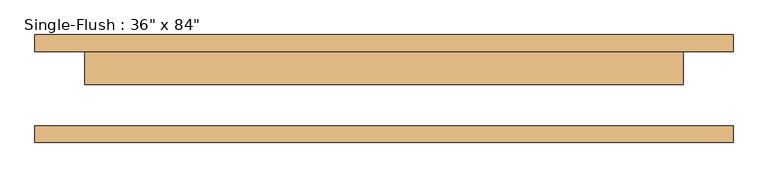
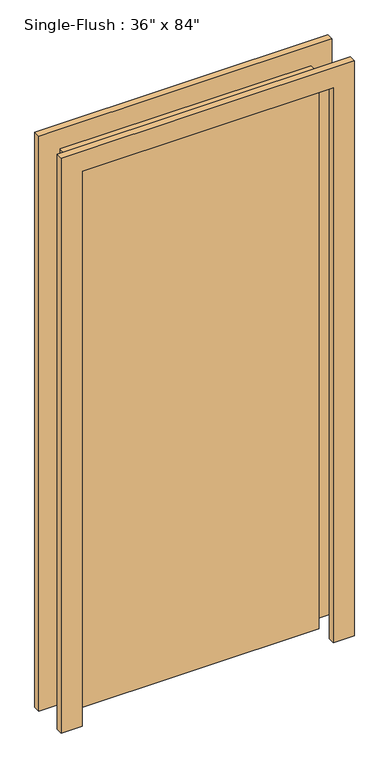
"""IFC4 building model written with IfcOpenShell, lengths in millimetres: door geometry."""

from ifc_helpers import new_model, si_unit, frame, origin, origin_with_axes, place, context, project, spatial, polyline, outline, extrude, source, transform, mapped, element, save


def door_e5f9f3c4(model_context):
    return source(origin(), model_context, "Body", "SweptSolid", [
        extrude(outline(polyline([(2209.8, -533.4), (0.0, -533.4), (0.0, -457.2), (2133.6, -457.2), (2133.6, 457.2), (0.0, 457.2), (0.0, 533.4), (2209.8, 533.4), (2209.8, -533.4)])), frame((0.0, 57.15, 0.0), z_axis=(0.0, 1.0, 0.0), x_axis=(0.0, 0.0, 1.0)), (0.0, 0.0, 1.0), 25.4),
        extrude(outline(polyline([(2209.8, 533.4), (2209.8, -533.4), (0.0, -533.4), (0.0, -457.2), (2133.6, -457.2), (2133.6, 457.2), (0.0, 457.2), (0.0, 533.4), (2209.8, 533.4)])), frame((0.0, -82.55, 0.0), z_axis=(0.0, 1.0, 0.0), x_axis=(0.0, 0.0, 1.0)), (0.0, 0.0, 1.0), 25.4),
        extrude(outline(polyline([(457.2, 6.35), (-457.2, 6.35), (-457.2, 57.15), (457.2, 57.15), (457.2, 6.35)])), origin_with_axes(), (0.0, 0.0, 1.0), 2133.6),
    ])


if __name__ == "__main__":
    model = new_model("IFC4")
    model_context = context("Model", 3, world=origin())
    ifc_project = project(units=[si_unit("LENGTHUNIT", "METRE", prefix="MILLI")], contexts=[model_context])
    site = spatial("IfcSite", under=ifc_project)
    building = spatial("IfcBuilding", under=site)
    placement = place(None, origin())
    door_shape = door_e5f9f3c4(model_context)
    element("IfcDoor", 1, ObjectType="Single-Flush : 36\" x 84\"", at=placement, inside=building, context=model_context, shape_type="MappedRepresentation", body=[
        mapped(door_shape, transform((0.0, 0.0, 0.0), x_axis=(1.0, 0.0, 0.0), y_axis=(0.0, 1.0, 0.0), z_axis=(0.0, 0.0, 1.0))),
    ])
    save(model, "model.ifc")

# Revit data of these elements
# Type "Single-Flush : 36\" x 84\""
#   Type Mark = "1"
#   Construction Type Id = "MDOOR"
#   Assembly Code = "C1020"
#   Analytic Construction = "Metal"
#   Thickness = 0' - 2"
#   Heat Transfer Coefficient (U) = 0.651978 BTU/(h·ft²·°F)
#   Height = 7' - 0"
#   Trim Projection Ext = 0' - 1"
#   Trim Projection Int = 0' - 1"
#   Trim Width = 0' - 3"
#   Width = 3' - 0"
#   Define Thermal Properties by = 1
#   Define Thermal Properties by = 1
#   Door Material = Door - Panel
#   Frame Material = Door - Frame
#   Visual Light Transmittance = 0
#   Solar Heat Gain Coefficient = 0
#   Function = (empty or 0)
#   Wall Closure = (empty or 0)
# Element 1 (IfcDoor, "Single-Flush : 36\" x 84\"")
#   Materials on its faces: "Door - Frame", "Door - Panel"
# Materials
#   "Door - Panel": class "Wood", colour RGB 210 159 95, transparency 0, Cost = 0
#   "Door - Frame": colour RGB 118 70 51, transparency 0, Cost = 0
